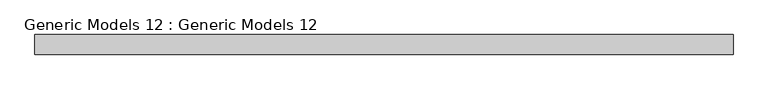
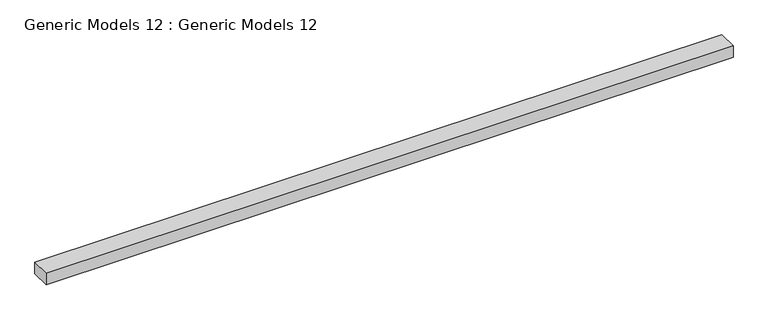
"""IFC4 building model written with IfcOpenShell, lengths in millimetres: proxy geometry, Generic Models 12 : Generic Models 12."""

from ifc_helpers import new_model, si_unit, frame, origin, place, context, project, spatial, polyline, outline, extrude, source, transform, mapped, element, save


def generic_models_12_generic_models_12_c9051349(model_context):
    return source(origin(), model_context, "Body", "SweptSolid", [
        extrude(outline(polyline([(3210.2495358, -21048.9985361), (-7649.2434833, -21048.9985361), (-7649.2434833, -20744.1985361), (3210.2495358, -20744.1985361), (3210.2495358, -21048.9985361)])), frame((0.0, 0.0, 2743.2), z_axis=(0.0, 0.0, 1.0), x_axis=(1.0, 0.0, 0.0)), (0.0, 0.0, 1.0), 191.1190684),
    ])


if __name__ == "__main__":
    model = new_model("IFC4")
    model_context = context("Model", 3, world=origin())
    ifc_project = project(units=[si_unit("LENGTHUNIT", "METRE", prefix="MILLI")], contexts=[model_context])
    site = spatial("IfcSite", under=ifc_project)
    building = spatial("IfcBuilding", under=site)
    placement = place(None, origin())
    generic_models_12_generic_models_12_shape = generic_models_12_generic_models_12_c9051349(model_context)
    element("IfcBuildingElementProxy", 1, Name="Generic Models 12 : Generic Models 12", ObjectType="Generic Models 12 : Generic Models 12", at=placement, inside=building, context=model_context, shape_type="MappedRepresentation", body=[
        mapped(generic_models_12_generic_models_12_shape, transform((0.0, 0.0, 0.0), x_axis=(1.0, 0.0, 0.0), y_axis=(0.0, 1.0, 0.0), z_axis=(0.0, 0.0, 1.0))),
    ])
    save(model, "model.ifc")
